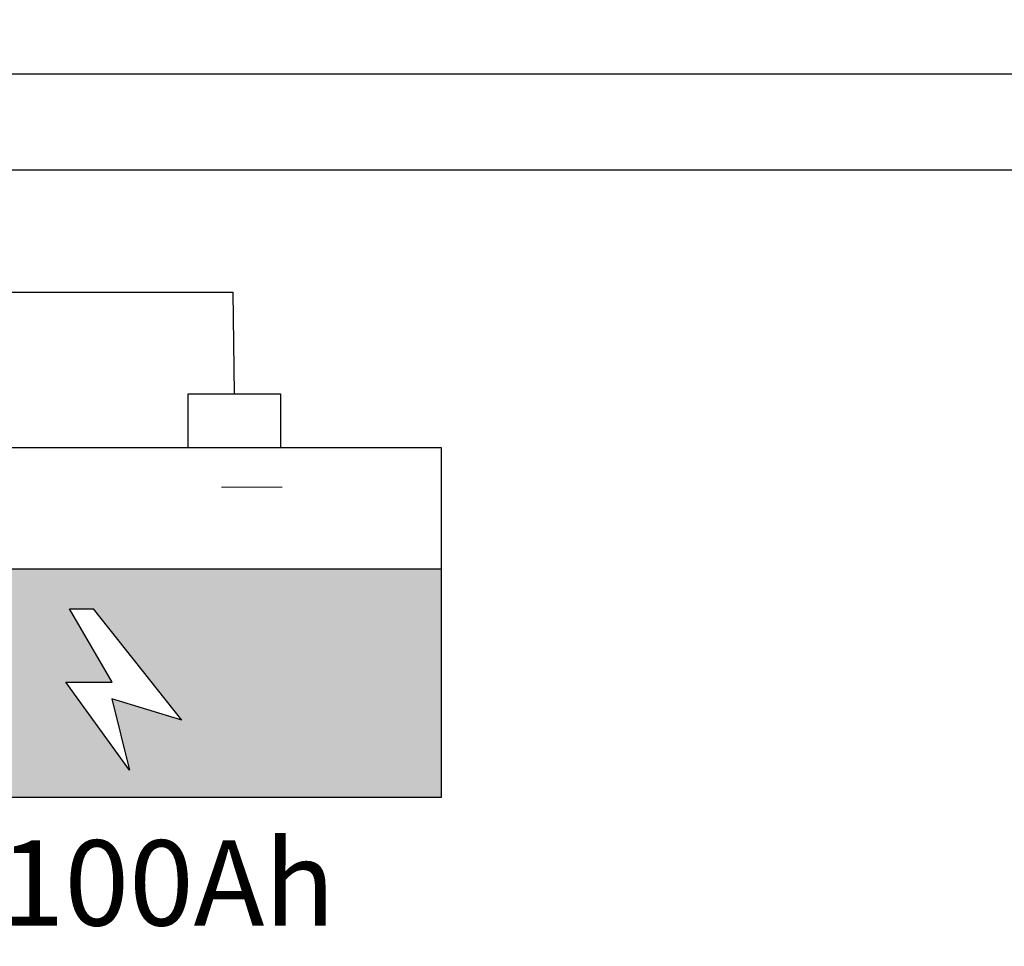
# Model space of a CAD drawing. Units: millimetres. Extents: x -8 to 285, y 5 to 221.
# Tile 8 of 30: x 84 to 130, y 13 to 56. Entities that reach past the tile are written whole.
import ezdxf

# ---------------------------------------------------------------- set-up
doc = ezdxf.new("R2010")
doc.units = ezdxf.units.MM
for name, color, linetype, lineweight in [('A-ANNO-DIMS', 2, 'Continuous', 18), ('E-ANNO-SYMB', 7, 'Continuous', 18), ('E-ANNO-TEXT', 7, 'Continuous', 18), ('E-EQPM-PATT', 252, 'Continuous', 13), ('E-POWR-BATT', 7, 'Continuous', 30), ('E-POWR-DC-NEG', 3, 'Continuous', 25)]:
    doc.layers.add(name, color=color, linetype=linetype, lineweight=lineweight)
doc.layers.add('E-POWR-DC-POS', color=30, linetype='Continuous', lineweight=25, true_color=0xf26722)
doc.styles.get("Standard").update_dxf_attribs({"font": 'arial.ttf'})
doc.dimstyles.get("Standard").update_dxf_attribs({"dimtxt": 0.18, "dimasz": 0.18, "dimexe": 0.18, "dimexo": 0.0625, "dimgap": 0.09, "dimtad": 0, "dimtih": 1, "dimtoh": 1, "dimdec": 4, "dimzin": 0, "dimdsep": 46, "dimtxsty": 'Standard', "dimcen": 0.09, "dimadec": 0, "dimazin": 0, "dimtfac": 1, "dimtdec": 4, "dimtofl": 0, "dimtmove": 0, "dimatfit": 3, "dimfxl": 1, "dimtolj": 1, "dimtzin": 0, "dimarcsym": 0})

# ---------------------------------------------------------------- blocks, each defined once
blk = doc.blocks.new('BATTERY-CASE')
blk.add_line((0, 10.738), (31.163, 10.738))
blk.add_lwpolyline([(0, 16.427), (31.163, 16.427), (31.163, 0), (0, 0)], close=True)
blk = doc.blocks.new('BATTERY-TERMINAL-POST')
for p, q in [((0, 0), (0, 2.525)), ((0, 2.525), (4.334, 2.525)), ((4.334, 2.525), (4.334, 0))]:
    blk.add_line(p, q)
blk = doc.blocks.new('BATTERY-LIGHTNING-EMBLEM')
for p, q in [((2.173, 4.126), (0.184, 7.57)), ((0.184, 7.57), (1.304, 7.57)), ((5.441, 2.343), (1.304, 7.57)), ((0, 4.126), (2.173, 4.126)), ((2.991, 0), (0, 4.126)), ((5.441, 2.343), (2.169, 3.351)), ((2.169, 3.351), (2.991, 0))]:
    blk.add_line(p, q)
blk = doc.blocks.new('*D10')
at = {"layer": 'A-ANNO-DIMS', "color": 0, "lineweight": -2, "transparency": 16777216}
for p, q in [((145.103, 206.457), (-7.608, 206.457)), ((-7.428, 206.277), (-7.428, 113.161)), ((-7.428, 19.682), (-7.428, 112.797)), ((30.453, 19.502), (-7.608, 19.502))]:
    blk.add_line(p, q, dxfattribs=at)
at = {"layer": 'A-ANNO-DIMS', "color": 0, "transparency": 16777216}
for points in [[(-7.458, 206.277), (-7.398, 206.277), (-7.428, 206.457)], [(-7.458, 19.682), (-7.398, 19.682), (-7.428, 19.502)]]:
    blk.add_solid(points, dxfattribs=at)
at = {"layer": 'Defpoints', "color": 0, "transparency": 16777216}
for p in [(-7.428, 206.457), (145.165, 206.457), (30.516, 19.502)]:
    blk.add_point(p, dxfattribs=at)
at = {"layer": 'A-ANNO-DIMS', "color": 0, "transparency": 16777216, "insert": (-7.428, 112.979), "char_height": 0.18, "attachment_point": 5}
blk.add_mtext('\\A1;186.95', dxfattribs=at)

msp = doc.modelspace()

# ---------------------------------------------------------------- hatches: boundary and pattern name
at = {"layer": 'E-EQPM-PATT'}
h = msp.add_hatch(color=256, dxfattribs=at)
h.set_gradient(color1=(244, 238, 81), color2=(248, 153, 30), tint=1)
h.paths.add_polyline_path([(30.516, 30.2396), (30.516, 19.502), (61.6786, 19.502), (61.6786, 30.2396)])
h.paths.add_polyline_path([(44.6613, 24.9143), (46.8335, 24.9143), (44.845, 28.3584), (45.9646, 28.3584), (50.1024, 23.1306), (46.8299, 24.1393), (47.652, 20.7882)], flags=16)
h.paths.add_polyline_path([(72.6568, 30.2396), (72.6568, 19.502), (103.8194, 19.502), (103.8194, 30.2396)])
h.paths.add_polyline_path([(86.2008, 24.9143), (88.373, 24.9143), (86.3846, 28.3584), (87.5041, 28.3584), (91.6419, 23.1306), (88.3694, 24.1393), (89.1915, 20.7882)], flags=16)

# ---------------------------------------------------------------- linework, layer by layer
at = {"layer": 'E-ANNO-SYMB'}
msp.add_line((93.5127, 34.0685), (96.3522, 34.0685), dxfattribs=at)
at = {"layer": 'E-POWR-DC-NEG'}
msp.add_line((58.1717, 53.4644), (215.8749, 53.4644), dxfattribs=at)
msp.add_lwpolyline([(58.1717, 67.9064), (58.1717, 43.2239), (94.0348, 43.2239), (94.1079, 38.4537)], dxfattribs=at)
at = {"layer": 'E-POWR-DC-POS'}
msp.add_lwpolyline([(52.1717, 48.962), (202.4345, 48.962), (202.4345, 34.9746)], dxfattribs=at)

# ---------------------------------------------------------------- block references
at = {"layer": 'E-POWR-BATT'}
for name, p in [('BATTERY-TERMINAL-POST', (91.9411, 35.929)), ('BATTERY-CASE', (72.6568, 19.502)), ('BATTERY-LIGHTNING-EMBLEM', (86.2005, 20.788))]:
    msp.add_blockref(name, p, dxfattribs=at)

# ---------------------------------------------------------------- texts
at = {"layer": 'E-ANNO-TEXT', "insert": (33.3813, 17.4943), "char_height": 4, "attachment_point": 1}
msp.add_mtext_dynamic_manual_height_columns('12V/100h            12V/100Ah', width=74.08228, gutter_width=12.5, heights=[0], dxfattribs=at)

# ---------------------------------------------------------------- dimensions: what is measured, and where the dimension line sits
at = {"layer": 'A-ANNO-DIMS'}
dim = msp.add_linear_dim(base=(-7.4275, 206.4568), p1=(30.516, 19.502), p2=(145.1651, 206.4568), angle=90, dimstyle='Standard', override={"dimdec": 2, "dimlfac": 1, "dimrnd": 0, "dimzin": 0, "dimdsep": 46, "dimlunit": 2}, dxfattribs=at)
dim.commit()
dim.dimension.update_dxf_attribs({"geometry": '*D10', "text_midpoint": (-7.4275, 112.9794)})

doc.saveas('drawing.dxf')
